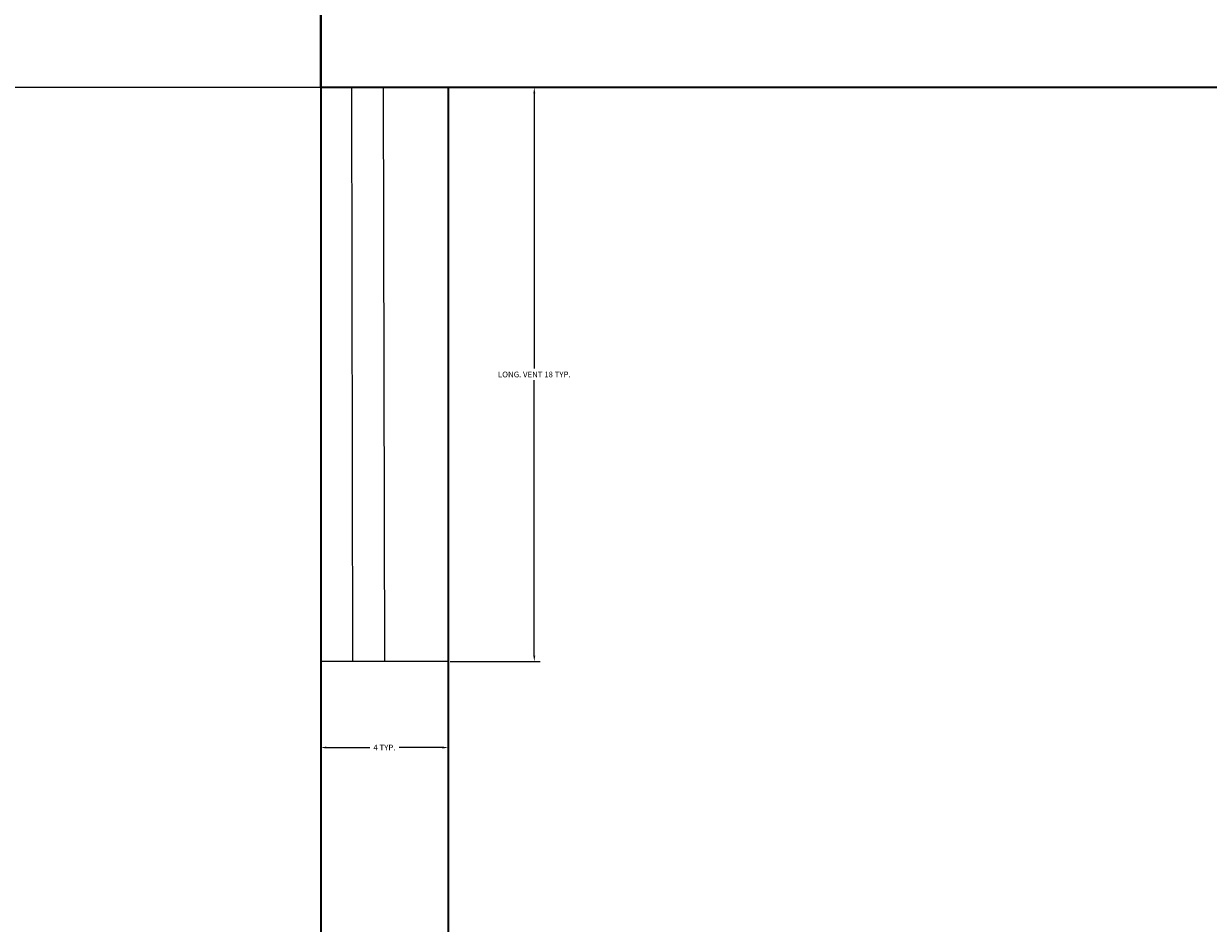
# Model space of a CAD drawing. Units: feet. Extents: x 105 to 1094, y -88 to 588.
# Tile 13 of 59: x 361 to 399, y 222 to 250. Entities that reach past the tile are written whole.
import ezdxf

# ---------------------------------------------------------------- set-up
doc = ezdxf.new("R2010")
doc.units = ezdxf.units.FT
doc.header["$MEASUREMENT"] = 0
for name, color, linetype, lineweight in [('A-ANNO-DIMS', 2, 'Continuous', 18), ('A-GLAZ', 4, 'Continuous', 18), ('A-WALL', 7, 'Continuous', 35)]:
    doc.layers.add(name, color=color, linetype=linetype, lineweight=lineweight)
doc.styles.get("Standard").update_dxf_attribs({"font": 'arial.ttf'})
doc.dimstyles.get("Standard").update_dxf_attribs({"dimtxt": 0.18, "dimasz": 0.18, "dimexe": 0.18, "dimexo": 0.0625, "dimgap": 0.09, "dimtad": 0, "dimtih": 1, "dimtoh": 1, "dimdec": 4, "dimzin": 0, "dimdsep": 46, "dimtxsty": 'Standard', "dimcen": 0.09, "dimadec": 0, "dimazin": 0, "dimtfac": 1, "dimtdec": 4, "dimtofl": 0, "dimtmove": 0, "dimatfit": 3, "dimfxl": 1, "dimtolj": 1, "dimtzin": 0, "dimarcsym": 0})

# ---------------------------------------------------------------- blocks, each defined once
blk = doc.blocks.new('VENT-LONGITUDINAL')
for p, q in [((0, 18), (4, 18)), ((2.039, 0), (2, 18)), ((3.039, 0.002), (3, 18.002))]:
    blk.add_line(p, q)
blk = doc.blocks.new('*D18')
at = {"layer": 'A-ANNO-DIMS', "color": 0, "lineweight": -2, "transparency": 16777216}
for p, q in [((374.751, 248.081), (377.569, 248.081)), ((377.389, 247.901), (377.389, 239.263)), ((377.389, 230.259), (377.389, 238.897)), ((374.751, 230.079), (377.569, 230.079))]:
    blk.add_line(p, q, dxfattribs=at)
at = {"layer": 'A-ANNO-DIMS', "color": 0, "transparency": 16777216}
for points in [[(377.359, 247.901), (377.419, 247.901), (377.389, 248.081)], [(377.359, 230.259), (377.419, 230.259), (377.389, 230.079)]]:
    blk.add_solid(points, dxfattribs=at)
at = {"layer": 'Defpoints', "color": 0, "transparency": 16777216}
for p in [(374.688, 248.081), (374.688, 230.079), (377.389, 230.079)]:
    blk.add_point(p, dxfattribs=at)
at = {"layer": 'A-ANNO-DIMS', "color": 0, "transparency": 16777216, "insert": (377.389, 239.08), "char_height": 0.18, "attachment_point": 5}
blk.add_mtext('\\A1;LONG. VENT 18 TYP.', dxfattribs=at)
blk = doc.blocks.new('*D19')
at = {"layer": 'A-ANNO-DIMS', "color": 0, "lineweight": -2, "transparency": 16777216}
for p, q in [((370.688, 230.016), (370.688, 227.199)), ((374.688, 230.016), (374.688, 227.199)), ((370.868, 227.379), (372.227, 227.379)), ((374.508, 227.379), (373.15, 227.379))]:
    blk.add_line(p, q, dxfattribs=at)
at = {"layer": 'A-ANNO-DIMS', "color": 0, "transparency": 16777216}
for points in [[(370.868, 227.409), (370.868, 227.349), (370.688, 227.379)], [(374.508, 227.409), (374.508, 227.349), (374.688, 227.379)]]:
    blk.add_solid(points, dxfattribs=at)
at = {"layer": 'Defpoints', "color": 0, "transparency": 16777216}
for p in [(370.688, 230.079), (374.688, 230.079), (370.688, 227.379)]:
    blk.add_point(p, dxfattribs=at)
at = {"layer": 'A-ANNO-DIMS', "color": 0, "transparency": 16777216, "insert": (372.688, 227.379), "char_height": 0.18, "attachment_point": 5}
blk.add_mtext('\\A1;4 TYP.', dxfattribs=at)
blk = doc.blocks.new('*D20')
at = {"layer": 'A-ANNO-DIMS', "color": 0, "lineweight": -2, "transparency": 16777216}
for p, q in [((150.688, 276.019), (150.688, -88.149)), ((1048.688, 276.019), (1048.688, -88.149)), ((150.868, -87.969), (599.399, -87.969)), ((1048.508, -87.969), (599.977, -87.969))]:
    blk.add_line(p, q, dxfattribs=at)
at = {"layer": 'A-ANNO-DIMS', "color": 0, "transparency": 16777216}
for points in [[(150.868, -87.939), (150.868, -87.999), (150.688, -87.969)], [(1048.508, -87.939), (1048.508, -87.999), (1048.688, -87.969)]]:
    blk.add_solid(points, dxfattribs=at)
at = {"layer": 'Defpoints', "color": 0, "transparency": 16777216}
for p in [(150.688, 276.081), (1048.688, 276.081), (1048.688, -87.969)]:
    blk.add_point(p, dxfattribs=at)
at = {"layer": 'A-ANNO-DIMS', "color": 0, "transparency": 16777216, "insert": (599.688, -87.969), "char_height": 0.18, "attachment_point": 5}
blk.add_mtext('\\A1;898', dxfattribs=at)
blk = doc.blocks.new('*D21')
at = {"layer": 'A-ANNO-DIMS', "color": 0, "lineweight": -2, "transparency": 16777216}
for p, q in [((849.626, 543.081), (105.458, 543.081)), ((105.638, 542.901), (105.638, 250.263)), ((105.638, -42.739), (105.638, 249.899)), ((849.626, -42.919), (105.458, -42.919))]:
    blk.add_line(p, q, dxfattribs=at)
at = {"layer": 'A-ANNO-DIMS', "color": 0, "transparency": 16777216}
for points in [[(105.608, 542.901), (105.668, 542.901), (105.638, 543.081)], [(105.608, -42.739), (105.668, -42.739), (105.638, -42.919)]]:
    blk.add_solid(points, dxfattribs=at)
at = {"layer": 'Defpoints', "color": 0, "transparency": 16777216}
for p in [(105.638, 543.081), (849.688, 543.081), (849.688, -42.919)]:
    blk.add_point(p, dxfattribs=at)
at = {"layer": 'A-ANNO-DIMS', "color": 0, "transparency": 16777216, "insert": (105.638, 250.081), "char_height": 0.18, "attachment_point": 5}
blk.add_mtext('\\A1;586', dxfattribs=at)
blk = doc.blocks.new('*D36')
at = {"layer": 'A-ANNO-DIMS', "color": 0, "lineweight": -2, "transparency": 16777216}
for p, q in [((547.235, 248.081), (105.458, 248.081)), ((105.638, 247.901), (105.638, 230.263)), ((105.638, 212.261), (105.638, 229.899)), ((546.626, 212.081), (105.458, 212.081))]:
    blk.add_line(p, q, dxfattribs=at)
at = {"layer": 'A-ANNO-DIMS', "color": 0, "transparency": 16777216}
for points in [[(105.608, 247.901), (105.668, 247.901), (105.638, 248.081)], [(105.608, 212.261), (105.668, 212.261), (105.638, 212.081)]]:
    blk.add_solid(points, dxfattribs=at)
at = {"layer": 'Defpoints', "color": 0, "transparency": 16777216}
for p in [(105.638, 248.081), (547.298, 248.081), (546.688, 212.081)]:
    blk.add_point(p, dxfattribs=at)
at = {"layer": 'A-ANNO-DIMS', "color": 0, "transparency": 16777216, "insert": (105.638, 230.081), "char_height": 0.18, "attachment_point": 5}
blk.add_mtext('\\A1;36', dxfattribs=at)
blk = doc.blocks.new('*D39')
at = {"layer": 'A-ANNO-DIMS', "color": 0, "lineweight": -2, "transparency": 16777216}
for p, q in [((294.688, 204.144), (294.688, 588.311)), ((370.688, 204.144), (370.688, 588.311)), ((294.868, 588.131), (332.47, 588.131)), ((370.508, 588.131), (332.906, 588.131))]:
    blk.add_line(p, q, dxfattribs=at)
at = {"layer": 'A-ANNO-DIMS', "color": 0, "transparency": 16777216}
for points in [[(294.868, 588.161), (294.868, 588.101), (294.688, 588.131)], [(370.508, 588.161), (370.508, 588.101), (370.688, 588.131)]]:
    blk.add_solid(points, dxfattribs=at)
at = {"layer": 'Defpoints', "color": 0, "transparency": 16777216}
for p in [(370.688, 588.131), (294.688, 204.081), (370.688, 204.081)]:
    blk.add_point(p, dxfattribs=at)
at = {"layer": 'A-ANNO-DIMS', "color": 0, "transparency": 16777216, "insert": (332.688, 588.131), "char_height": 0.18, "attachment_point": 5}
blk.add_mtext('\\A1;76', dxfattribs=at)

msp = doc.modelspace()

# ---------------------------------------------------------------- linework, layer by layer
at = {"layer": 'A-WALL'}
for p, q in [((370.6883, 248.0812), (370.6883, 296.0812)), ((370.6883, 252.0812), (370.6883, 204.0812)), ((552.6883, 248.0812), (370.6883, 248.0812)), ((422.6883, 248.0812), (370.6883, 248.0812)), ((374.6883, 248.0812), (374.6883, 146.0812))]:
    msp.add_line(p, q, dxfattribs=at)

# ---------------------------------------------------------------- block references
at = {"layer": 'A-GLAZ', "rotation": 180}
msp.add_blockref('VENT-LONGITUDINAL', (374.6886, 248.0813), dxfattribs=at)

# ---------------------------------------------------------------- dimensions: what is measured, and where the dimension line sits
at = {"layer": 'A-ANNO-DIMS'}
for base, p1, p2, picture, middle in [((370.6883, 588.1312), (294.6883, 204.0812), (370.6883, 204.0812), '*D39', (332.6883, 588.1312)), ((1048.6883, -87.9688), (150.6883, 276.0812), (1048.6883, 276.0812), '*D20', (599.6883, -87.9688))]:
    dim = msp.add_linear_dim(base=base, p1=p1, p2=p2, dimstyle='Standard', override={"dimdec": 0, "dimlfac": 1, "dimrnd": 0, "dimzin": 0, "dimdsep": 46, "dimlunit": 2}, dxfattribs=at)
    dim.commit()
    dim.dimension.update_dxf_attribs({"geometry": picture, "text_midpoint": middle})
for base, p1, p2, picture, middle in [((105.6383, 543.0812), (849.6883, -42.9188), (849.6883, 543.0812), '*D21', (105.6383, 250.0812)), ((105.6383, 248.0812), (546.6883, 212.0812), (547.2975, 248.0812), '*D36', (105.6383, 230.0812))]:
    dim = msp.add_linear_dim(base=base, p1=p1, p2=p2, angle=90, dimstyle='Standard', override={"dimdec": 0, "dimlfac": 1, "dimrnd": 0, "dimzin": 0, "dimdsep": 46, "dimlunit": 2}, dxfattribs=at)
    dim.commit()
    dim.dimension.update_dxf_attribs({"geometry": picture, "text_midpoint": middle})
for base, p1, p2, angle, text, picture, middle in [((377.3886, 230.079), (374.6883, 248.0812), (374.6883, 230.079), 270, 'LONG. VENT <> TYP.', '*D18', (377.3886, 239.0801)), ((370.6883, 227.3787), (374.6883, 230.079), (370.6883, 230.079), 180, '<> TYP.', '*D19', (372.6883, 227.3787))]:
    dim = msp.add_linear_dim(base=base, p1=p1, p2=p2, angle=angle, text=text, dimstyle='Standard', override={"dimdec": 0, "dimlfac": 1, "dimrnd": 0, "dimzin": 0, "dimdsep": 46, "dimlunit": 2}, dxfattribs=at)
    dim.commit()
    dim.dimension.update_dxf_attribs({"geometry": picture, "text_midpoint": middle})

doc.saveas('drawing.dxf')
